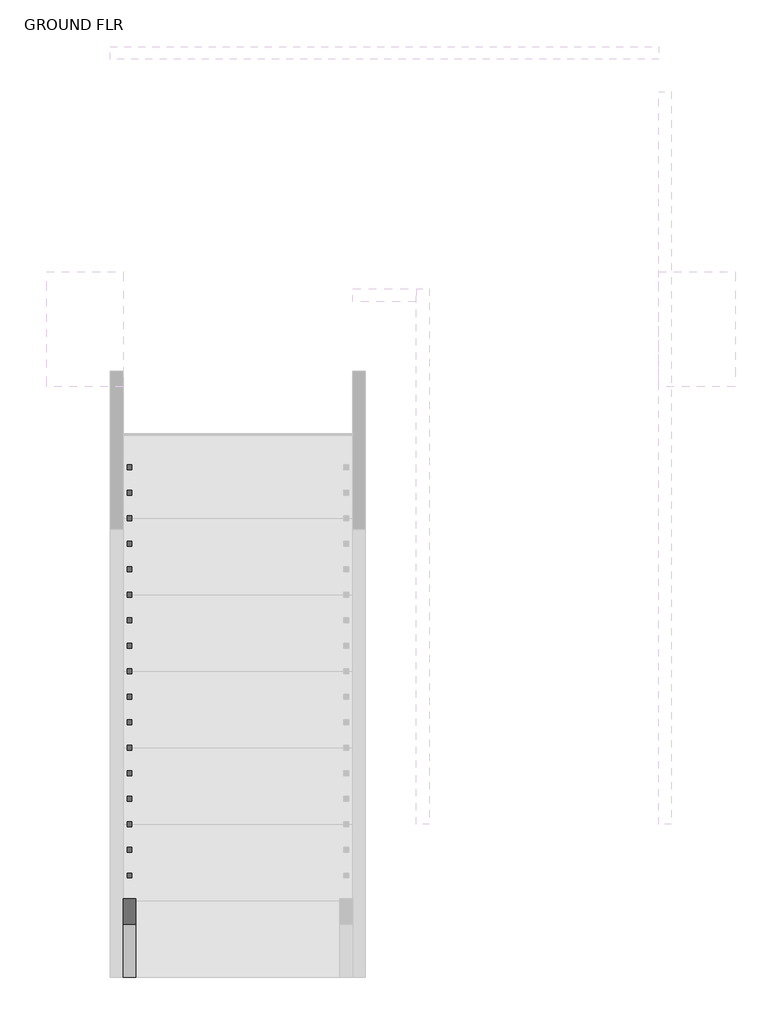
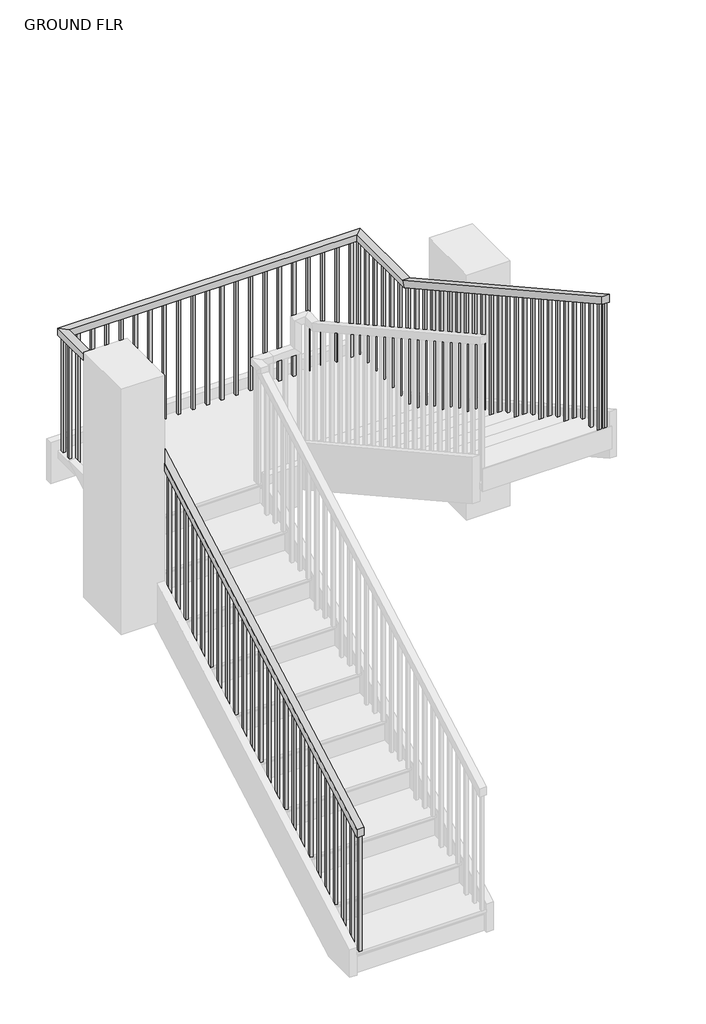
# One storey, part 2 of 4: 1 railing.
"""IFC4 building model written with IfcOpenShell, lengths in millimetres."""

from ifc_helpers import new_model, si_unit, frame, origin, place, context, project, spatial, polyline, outline, extrude, faceted_brep, element, save

model = new_model("IFC4")

# Units and contexts
model_context = context("Model", 3, world=origin())
ifc_project = project(units=[si_unit("LENGTHUNIT", "METRE", prefix="MILLI")], contexts=[model_context])

# Site, building, storey
site = spatial("IfcSite", under=ifc_project)
building = spatial("IfcBuilding", under=site)
storey = spatial("IfcBuildingStorey", under=building, Name="GROUND FLR", Elevation=304.8)

# Railing
placement = place(None, origin())
element("IfcRailing", 1, ObjectType="Handrail - Rectangular", at=placement, inside=storey, context=model_context, shape_type="SolidModel", body=[
    faceted_brep([(-992.1175798, -12221.8061634, 1388.5333333), (-992.1175798, -12221.8061634, 1330.420221), (-941.3175798, -12221.8061634, 1330.420221), (-941.3175798, -12221.8061634, 1388.5333333), (-992.1175798, -9478.6061634, 2912.5333333), (-992.1175798, -9465.4425611, 2861.7333333), (-941.3175798, -9465.4425611, 2861.7333333), (-941.3175798, -9478.6061634, 2912.5333333), (-992.1175798, -8564.2061634, 2912.5333333), (-992.1175798, -8564.2061634, 2861.7333333), (-941.3175798, -8615.0061634, 2861.7333333), (-941.3175798, -8615.0061634, 2912.5333333), (1141.4824202, -8564.2061634, 2912.5333333), (1141.4824202, -8564.2061634, 2861.7333333), (1090.6824202, -8615.0061634, 2861.7333333), (1090.6824202, -8615.0061634, 2912.5333333), (1141.4824202, -9173.8061634, 2912.5333333), (1141.4824202, -9186.9697656, 2861.7333333), (1090.6824202, -9186.9697656, 2861.7333333), (1090.6824202, -9173.8061634, 2912.5333333), (1141.4824202, -11612.2061634, 4267.2), (1090.6824202, -11612.2061634, 4267.2), (1090.6824202, -11612.2061634, 4209.0868876), (1141.4824202, -11612.2061634, 4209.0868876)], [[[0, 1, 2, 3]], [[1, 0, 4, 5]], [[2, 1, 5, 6]], [[3, 2, 6, 7]], [[0, 3, 7, 4]], [[5, 4, 8, 9]], [[6, 5, 9, 10]], [[7, 6, 10, 11]], [[4, 7, 11, 8]], [[9, 8, 12, 13]], [[10, 9, 13, 14]], [[11, 10, 14, 15]], [[8, 11, 15, 12]], [[13, 12, 16, 17]], [[14, 13, 17, 18]], [[15, 14, 18, 19]], [[12, 15, 19, 16]], [[20, 21, 22, 23]], [[17, 16, 20, 23]], [[18, 17, 23, 22]], [[19, 18, 22, 21]], [[16, 19, 21, 20]]]),
    extrude(outline(polyline([(-11526.4811634, 4161.4618876), (-11526.4811634, 3183.4666667), (-11545.5311634, 3183.4666667), (-11545.5311634, 4172.045221), (-11526.4811634, 4161.4618876)])), frame((1106.5574202, 0.0, 0.0), z_axis=(1.0, 0.0, 0.0), x_axis=(0.0, 1.0, 0.0)), (0.0, 0.0, 1.0), 19.05),
    extrude(outline(polyline([(-11424.8811634, 4105.0174432), (-11424.8811634, 3183.4666667), (-11443.9311634, 3183.4666667), (-11443.9311634, 4115.6007765), (-11424.8811634, 4105.0174432)])), frame((1106.5574202, 0.0, 0.0), z_axis=(1.0, 0.0, 0.0), x_axis=(0.0, 1.0, 0.0)), (0.0, 0.0, 1.0), 19.05),
    extrude(outline(polyline([(-11323.2811634, 4048.5729988), (-11323.2811634, 3183.4666667), (-11342.3311634, 3183.4666667), (-11342.3311634, 4059.1563321), (-11323.2811634, 4048.5729988)])), frame((1106.5574202, 0.0, 0.0), z_axis=(1.0, 0.0, 0.0), x_axis=(0.0, 1.0, 0.0)), (0.0, 0.0, 1.0), 19.05),
    extrude(outline(polyline([(-11221.6811634, 3992.1285543), (-11221.6811634, 3014.1333333), (-11240.7311634, 3014.1333333), (-11240.7311634, 4002.7118876), (-11221.6811634, 3992.1285543)])), frame((1106.5574202, 0.0, 0.0), z_axis=(1.0, 0.0, 0.0), x_axis=(0.0, 1.0, 0.0)), (0.0, 0.0, 1.0), 19.05),
    extrude(outline(polyline([(-11120.0811634, 3935.6841099), (-11120.0811634, 3014.1333333), (-11139.1311634, 3014.1333333), (-11139.1311634, 3946.2674432), (-11120.0811634, 3935.6841099)])), frame((1106.5574202, 0.0, 0.0), z_axis=(1.0, 0.0, 0.0), x_axis=(0.0, 1.0, 0.0)), (0.0, 0.0, 1.0), 19.05),
    extrude(outline(polyline([(-11018.4811634, 3879.2396654), (-11018.4811634, 3014.1333333), (-11037.5311634, 3014.1333333), (-11037.5311634, 3889.8229988), (-11018.4811634, 3879.2396654)])), frame((1106.5574202, 0.0, 0.0), z_axis=(1.0, 0.0, 0.0), x_axis=(0.0, 1.0, 0.0)), (0.0, 0.0, 1.0), 19.05),
    extrude(outline(polyline([(-10916.8811634, 3822.795221), (-10916.8811634, 2844.8), (-10935.9311634, 2844.8), (-10935.9311634, 3833.3785543), (-10916.8811634, 3822.795221)])), frame((1106.5574202, 0.0, 0.0), z_axis=(1.0, 0.0, 0.0), x_axis=(0.0, 1.0, 0.0)), (0.0, 0.0, 1.0), 19.05),
    extrude(outline(polyline([(-10815.2811634, 3766.3507765), (-10815.2811634, 2844.8), (-10834.3311634, 2844.8), (-10834.3311634, 3776.9341099), (-10815.2811634, 3766.3507765)])), frame((1106.5574202, 0.0, 0.0), z_axis=(1.0, 0.0, 0.0), x_axis=(0.0, 1.0, 0.0)), (0.0, 0.0, 1.0), 19.05),
    extrude(outline(polyline([(-10713.6811634, 3709.9063321), (-10713.6811634, 2844.8), (-10732.7311634, 2844.8), (-10732.7311634, 3720.4896654), (-10713.6811634, 3709.9063321)])), frame((1106.5574202, 0.0, 0.0), z_axis=(1.0, 0.0, 0.0), x_axis=(0.0, 1.0, 0.0)), (0.0, 0.0, 1.0), 19.05),
    extrude(outline(polyline([(-10612.0811634, 3653.4618876), (-10612.0811634, 2675.4666667), (-10631.1311634, 2675.4666667), (-10631.1311634, 3664.045221), (-10612.0811634, 3653.4618876)])), frame((1106.5574202, 0.0, 0.0), z_axis=(1.0, 0.0, 0.0), x_axis=(0.0, 1.0, 0.0)), (0.0, 0.0, 1.0), 19.05),
    extrude(outline(polyline([(-10510.4811634, 3597.0174432), (-10510.4811634, 2675.4666667), (-10529.5311634, 2675.4666667), (-10529.5311634, 3607.6007765), (-10510.4811634, 3597.0174432)])), frame((1106.5574202, 0.0, 0.0), z_axis=(1.0, 0.0, 0.0), x_axis=(0.0, 1.0, 0.0)), (0.0, 0.0, 1.0), 19.05),
    extrude(outline(polyline([(-10408.8811634, 3540.5729988), (-10408.8811634, 2675.4666667), (-10427.9311634, 2675.4666667), (-10427.9311634, 3551.1563321), (-10408.8811634, 3540.5729988)])), frame((1106.5574202, 0.0, 0.0), z_axis=(1.0, 0.0, 0.0), x_axis=(0.0, 1.0, 0.0)), (0.0, 0.0, 1.0), 19.05),
    extrude(outline(polyline([(-10307.2811634, 3484.1285543), (-10307.2811634, 2506.1333333), (-10326.3311634, 2506.1333333), (-10326.3311634, 3494.7118876), (-10307.2811634, 3484.1285543)])), frame((1106.5574202, 0.0, 0.0), z_axis=(1.0, 0.0, 0.0), x_axis=(0.0, 1.0, 0.0)), (0.0, 0.0, 1.0), 19.05),
    extrude(outline(polyline([(-10205.6811634, 3427.6841099), (-10205.6811634, 2506.1333333), (-10224.7311634, 2506.1333333), (-10224.7311634, 3438.2674432), (-10205.6811634, 3427.6841099)])), frame((1106.5574202, 0.0, 0.0), z_axis=(1.0, 0.0, 0.0), x_axis=(0.0, 1.0, 0.0)), (0.0, 0.0, 1.0), 19.05),
    extrude(outline(polyline([(-10104.0811634, 3371.2396654), (-10104.0811634, 2506.1333333), (-10123.1311634, 2506.1333333), (-10123.1311634, 3381.8229988), (-10104.0811634, 3371.2396654)])), frame((1106.5574202, 0.0, 0.0), z_axis=(1.0, 0.0, 0.0), x_axis=(0.0, 1.0, 0.0)), (0.0, 0.0, 1.0), 19.05),
    extrude(outline(polyline([(-10002.4811634, 3314.795221), (-10002.4811634, 2336.8), (-10021.5311634, 2336.8), (-10021.5311634, 3325.3785543), (-10002.4811634, 3314.795221)])), frame((1106.5574202, 0.0, 0.0), z_axis=(1.0, 0.0, 0.0), x_axis=(0.0, 1.0, 0.0)), (0.0, 0.0, 1.0), 19.05),
    extrude(outline(polyline([(-9900.8811634, 3258.3507765), (-9900.8811634, 2336.8), (-9919.9311634, 2336.8), (-9919.9311634, 3268.9341099), (-9900.8811634, 3258.3507765)])), frame((1106.5574202, 0.0, 0.0), z_axis=(1.0, 0.0, 0.0), x_axis=(0.0, 1.0, 0.0)), (0.0, 0.0, 1.0), 19.05),
    extrude(outline(polyline([(-9799.2811634, 3201.9063321), (-9799.2811634, 2336.8), (-9818.3311634, 2336.8), (-9818.3311634, 3212.4896654), (-9799.2811634, 3201.9063321)])), frame((1106.5574202, 0.0, 0.0), z_axis=(1.0, 0.0, 0.0), x_axis=(0.0, 1.0, 0.0)), (0.0, 0.0, 1.0), 19.05),
    extrude(outline(polyline([(-9697.6811634, 3145.4618876), (-9697.6811634, 2167.4666667), (-9716.7311634, 2167.4666667), (-9716.7311634, 3156.045221), (-9697.6811634, 3145.4618876)])), frame((1106.5574202, 0.0, 0.0), z_axis=(1.0, 0.0, 0.0), x_axis=(0.0, 1.0, 0.0)), (0.0, 0.0, 1.0), 19.05),
    extrude(outline(polyline([(-9596.0811634, 3089.0174432), (-9596.0811634, 2167.4666667), (-9615.1311634, 2167.4666667), (-9615.1311634, 3099.6007765), (-9596.0811634, 3089.0174432)])), frame((1106.5574202, 0.0, 0.0), z_axis=(1.0, 0.0, 0.0), x_axis=(0.0, 1.0, 0.0)), (0.0, 0.0, 1.0), 19.05),
    extrude(outline(polyline([(-9494.4811634, 3032.5729988), (-9494.4811634, 2167.4666667), (-9513.5311634, 2167.4666667), (-9513.5311634, 3043.1563321), (-9494.4811634, 3032.5729988)])), frame((1106.5574202, 0.0, 0.0), z_axis=(1.0, 0.0, 0.0), x_axis=(0.0, 1.0, 0.0)), (0.0, 0.0, 1.0), 19.05),
    extrude(outline(polyline([(-9392.8811634, 2976.1285543), (-9392.8811634, 1998.1333333), (-9411.9311634, 1998.1333333), (-9411.9311634, 2986.7118876), (-9392.8811634, 2976.1285543)])), frame((1106.5574202, 0.0, 0.0), z_axis=(1.0, 0.0, 0.0), x_axis=(0.0, 1.0, 0.0)), (0.0, 0.0, 1.0), 19.05),
    extrude(outline(polyline([(-9291.2811634, 2919.6841099), (-9291.2811634, 1998.1333333), (-9310.3311634, 1998.1333333), (-9310.3311634, 2930.2674432), (-9291.2811634, 2919.6841099)])), frame((1106.5574202, 0.0, 0.0), z_axis=(1.0, 0.0, 0.0), x_axis=(0.0, 1.0, 0.0)), (0.0, 0.0, 1.0), 19.05),
    extrude(outline(polyline([(-9189.6811634, 2863.2396654), (-9189.6811634, 1998.1333333), (-9208.7311634, 1998.1333333), (-9208.7311634, 2873.8229988), (-9189.6811634, 2863.2396654)])), frame((1106.5574202, 0.0, 0.0), z_axis=(1.0, 0.0, 0.0), x_axis=(0.0, 1.0, 0.0)), (0.0, 0.0, 1.0), 19.05),
    extrude(outline(polyline([(1125.6074202, -9088.0811634), (1125.6074202, -9107.1311634), (1106.5574202, -9107.1311634), (1106.5574202, -9088.0811634), (1125.6074202, -9088.0811634)])), frame((0.0, 0.0, 1998.1333333), z_axis=(0.0, 0.0, 1.0), x_axis=(1.0, 0.0, 0.0)), (0.0, 0.0, 1.0), 863.6),
    extrude(outline(polyline([(1125.6074202, -8986.4811634), (1125.6074202, -9005.5311634), (1106.5574202, -9005.5311634), (1106.5574202, -8986.4811634), (1125.6074202, -8986.4811634)])), frame((0.0, 0.0, 1998.1333333), z_axis=(0.0, 0.0, 1.0), x_axis=(1.0, 0.0, 0.0)), (0.0, 0.0, 1.0), 863.6),
    extrude(outline(polyline([(1125.6074202, -8884.8811634), (1125.6074202, -8903.9311634), (1106.5574202, -8903.9311634), (1106.5574202, -8884.8811634), (1125.6074202, -8884.8811634)])), frame((0.0, 0.0, 1998.1333333), z_axis=(0.0, 0.0, 1.0), x_axis=(1.0, 0.0, 0.0)), (0.0, 0.0, 1.0), 863.6),
    extrude(outline(polyline([(1125.6074202, -8783.2811634), (1125.6074202, -8802.3311634), (1106.5574202, -8802.3311634), (1106.5574202, -8783.2811634), (1125.6074202, -8783.2811634)])), frame((0.0, 0.0, 1998.1333333), z_axis=(0.0, 0.0, 1.0), x_axis=(1.0, 0.0, 0.0)), (0.0, 0.0, 1.0), 863.6),
    extrude(outline(polyline([(1125.6074202, -8681.6811634), (1125.6074202, -8700.7311634), (1106.5574202, -8700.7311634), (1106.5574202, -8681.6811634), (1125.6074202, -8681.6811634)])), frame((0.0, 0.0, 1998.1333333), z_axis=(0.0, 0.0, 1.0), x_axis=(1.0, 0.0, 0.0)), (0.0, 0.0, 1.0), 863.6),
    extrude(outline(polyline([(1055.7574202, -8580.0811634), (1074.8074202, -8580.0811634), (1074.8074202, -8599.1311634), (1055.7574202, -8599.1311634), (1055.7574202, -8580.0811634)])), frame((0.0, 0.0, 1998.1333333), z_axis=(0.0, 0.0, 1.0), x_axis=(1.0, 0.0, 0.0)), (0.0, 0.0, 1.0), 863.6),
    extrude(outline(polyline([(954.1574202, -8580.0811634), (973.2074202, -8580.0811634), (973.2074202, -8599.1311634), (954.1574202, -8599.1311634), (954.1574202, -8580.0811634)])), frame((0.0, 0.0, 1998.1333333), z_axis=(0.0, 0.0, 1.0), x_axis=(1.0, 0.0, 0.0)), (0.0, 0.0, 1.0), 863.6),
    extrude(outline(polyline([(852.5574202, -8580.0811634), (871.6074202, -8580.0811634), (871.6074202, -8599.1311634), (852.5574202, -8599.1311634), (852.5574202, -8580.0811634)])), frame((0.0, 0.0, 1998.1333333), z_axis=(0.0, 0.0, 1.0), x_axis=(1.0, 0.0, 0.0)), (0.0, 0.0, 1.0), 863.6),
    extrude(outline(polyline([(750.9574202, -8580.0811634), (770.0074202, -8580.0811634), (770.0074202, -8599.1311634), (750.9574202, -8599.1311634), (750.9574202, -8580.0811634)])), frame((0.0, 0.0, 1998.1333333), z_axis=(0.0, 0.0, 1.0), x_axis=(1.0, 0.0, 0.0)), (0.0, 0.0, 1.0), 863.6),
    extrude(outline(polyline([(649.3574202, -8580.0811634), (668.4074202, -8580.0811634), (668.4074202, -8599.1311634), (649.3574202, -8599.1311634), (649.3574202, -8580.0811634)])), frame((0.0, 0.0, 1998.1333333), z_axis=(0.0, 0.0, 1.0), x_axis=(1.0, 0.0, 0.0)), (0.0, 0.0, 1.0), 863.6),
    extrude(outline(polyline([(547.7574202, -8580.0811634), (566.8074202, -8580.0811634), (566.8074202, -8599.1311634), (547.7574202, -8599.1311634), (547.7574202, -8580.0811634)])), frame((0.0, 0.0, 1998.1333333), z_axis=(0.0, 0.0, 1.0), x_axis=(1.0, 0.0, 0.0)), (0.0, 0.0, 1.0), 863.6),
    extrude(outline(polyline([(446.1574202, -8580.0811634), (465.2074202, -8580.0811634), (465.2074202, -8599.1311634), (446.1574202, -8599.1311634), (446.1574202, -8580.0811634)])), frame((0.0, 0.0, 1998.1333333), z_axis=(0.0, 0.0, 1.0), x_axis=(1.0, 0.0, 0.0)), (0.0, 0.0, 1.0), 863.6),
    extrude(outline(polyline([(344.5574202, -8580.0811634), (363.6074202, -8580.0811634), (363.6074202, -8599.1311634), (344.5574202, -8599.1311634), (344.5574202, -8580.0811634)])), frame((0.0, 0.0, 1998.1333333), z_axis=(0.0, 0.0, 1.0), x_axis=(1.0, 0.0, 0.0)), (0.0, 0.0, 1.0), 863.6),
    extrude(outline(polyline([(242.9574202, -8580.0811634), (262.0074202, -8580.0811634), (262.0074202, -8599.1311634), (242.9574202, -8599.1311634), (242.9574202, -8580.0811634)])), frame((0.0, 0.0, 1998.1333333), z_axis=(0.0, 0.0, 1.0), x_axis=(1.0, 0.0, 0.0)), (0.0, 0.0, 1.0), 863.6),
    extrude(outline(polyline([(141.3574202, -8580.0811634), (160.4074202, -8580.0811634), (160.4074202, -8599.1311634), (141.3574202, -8599.1311634), (141.3574202, -8580.0811634)])), frame((0.0, 0.0, 1998.1333333), z_axis=(0.0, 0.0, 1.0), x_axis=(1.0, 0.0, 0.0)), (0.0, 0.0, 1.0), 863.6),
    extrude(outline(polyline([(39.7574202, -8580.0811634), (58.8074202, -8580.0811634), (58.8074202, -8599.1311634), (39.7574202, -8599.1311634), (39.7574202, -8580.0811634)])), frame((0.0, 0.0, 1998.1333333), z_axis=(0.0, 0.0, 1.0), x_axis=(1.0, 0.0, 0.0)), (0.0, 0.0, 1.0), 863.6),
    extrude(outline(polyline([(-61.8425798, -8580.0811634), (-42.7925798, -8580.0811634), (-42.7925798, -8599.1311634), (-61.8425798, -8599.1311634), (-61.8425798, -8580.0811634)])), frame((0.0, 0.0, 1998.1333333), z_axis=(0.0, 0.0, 1.0), x_axis=(1.0, 0.0, 0.0)), (0.0, 0.0, 1.0), 863.6),
    extrude(outline(polyline([(-163.4425798, -8580.0811634), (-144.3925798, -8580.0811634), (-144.3925798, -8599.1311634), (-163.4425798, -8599.1311634), (-163.4425798, -8580.0811634)])), frame((0.0, 0.0, 1998.1333333), z_axis=(0.0, 0.0, 1.0), x_axis=(1.0, 0.0, 0.0)), (0.0, 0.0, 1.0), 863.6),
    extrude(outline(polyline([(-265.0425798, -8580.0811634), (-245.9925798, -8580.0811634), (-245.9925798, -8599.1311634), (-265.0425798, -8599.1311634), (-265.0425798, -8580.0811634)])), frame((0.0, 0.0, 1998.1333333), z_axis=(0.0, 0.0, 1.0), x_axis=(1.0, 0.0, 0.0)), (0.0, 0.0, 1.0), 863.6),
    extrude(outline(polyline([(-366.6425798, -8580.0811634), (-347.5925798, -8580.0811634), (-347.5925798, -8599.1311634), (-366.6425798, -8599.1311634), (-366.6425798, -8580.0811634)])), frame((0.0, 0.0, 1998.1333333), z_axis=(0.0, 0.0, 1.0), x_axis=(1.0, 0.0, 0.0)), (0.0, 0.0, 1.0), 863.6),
    extrude(outline(polyline([(-468.2425798, -8580.0811634), (-449.1925798, -8580.0811634), (-449.1925798, -8599.1311634), (-468.2425798, -8599.1311634), (-468.2425798, -8580.0811634)])), frame((0.0, 0.0, 1998.1333333), z_axis=(0.0, 0.0, 1.0), x_axis=(1.0, 0.0, 0.0)), (0.0, 0.0, 1.0), 863.6),
    extrude(outline(polyline([(-569.8425798, -8580.0811634), (-550.7925798, -8580.0811634), (-550.7925798, -8599.1311634), (-569.8425798, -8599.1311634), (-569.8425798, -8580.0811634)])), frame((0.0, 0.0, 1998.1333333), z_axis=(0.0, 0.0, 1.0), x_axis=(1.0, 0.0, 0.0)), (0.0, 0.0, 1.0), 863.6),
    extrude(outline(polyline([(-671.4425798, -8580.0811634), (-652.3925798, -8580.0811634), (-652.3925798, -8599.1311634), (-671.4425798, -8599.1311634), (-671.4425798, -8580.0811634)])), frame((0.0, 0.0, 1998.1333333), z_axis=(0.0, 0.0, 1.0), x_axis=(1.0, 0.0, 0.0)), (0.0, 0.0, 1.0), 863.6),
    extrude(outline(polyline([(-773.0425798, -8580.0811634), (-753.9925798, -8580.0811634), (-753.9925798, -8599.1311634), (-773.0425798, -8599.1311634), (-773.0425798, -8580.0811634)])), frame((0.0, 0.0, 1998.1333333), z_axis=(0.0, 0.0, 1.0), x_axis=(1.0, 0.0, 0.0)), (0.0, 0.0, 1.0), 863.6),
    extrude(outline(polyline([(-874.6425798, -8580.0811634), (-855.5925798, -8580.0811634), (-855.5925798, -8599.1311634), (-874.6425798, -8599.1311634), (-874.6425798, -8580.0811634)])), frame((0.0, 0.0, 1998.1333333), z_axis=(0.0, 0.0, 1.0), x_axis=(1.0, 0.0, 0.0)), (0.0, 0.0, 1.0), 863.6),
    extrude(outline(polyline([(-976.2425798, -8675.3311634), (-976.2425798, -8656.2811634), (-957.1925798, -8656.2811634), (-957.1925798, -8675.3311634), (-976.2425798, -8675.3311634)])), frame((0.0, 0.0, 1998.1333333), z_axis=(0.0, 0.0, 1.0), x_axis=(1.0, 0.0, 0.0)), (0.0, 0.0, 1.0), 863.6),
    extrude(outline(polyline([(-976.2425798, -8776.9311634), (-976.2425798, -8757.8811634), (-957.1925798, -8757.8811634), (-957.1925798, -8776.9311634), (-976.2425798, -8776.9311634)])), frame((0.0, 0.0, 1998.1333333), z_axis=(0.0, 0.0, 1.0), x_axis=(1.0, 0.0, 0.0)), (0.0, 0.0, 1.0), 863.6),
    extrude(outline(polyline([(-976.2425798, -8878.5311634), (-976.2425798, -8859.4811634), (-957.1925798, -8859.4811634), (-957.1925798, -8878.5311634), (-976.2425798, -8878.5311634)])), frame((0.0, 0.0, 1998.1333333), z_axis=(0.0, 0.0, 1.0), x_axis=(1.0, 0.0, 0.0)), (0.0, 0.0, 1.0), 863.6),
    extrude(outline(polyline([(-976.2425798, -8980.1311634), (-976.2425798, -8961.0811634), (-957.1925798, -8961.0811634), (-957.1925798, -8980.1311634), (-976.2425798, -8980.1311634)])), frame((0.0, 0.0, 1998.1333333), z_axis=(0.0, 0.0, 1.0), x_axis=(1.0, 0.0, 0.0)), (0.0, 0.0, 1.0), 863.6),
    extrude(outline(polyline([(-976.2425798, -9081.7311634), (-976.2425798, -9062.6811634), (-957.1925798, -9062.6811634), (-957.1925798, -9081.7311634), (-976.2425798, -9081.7311634)])), frame((0.0, 0.0, 1998.1333333), z_axis=(0.0, 0.0, 1.0), x_axis=(1.0, 0.0, 0.0)), (0.0, 0.0, 1.0), 863.6),
    extrude(outline(polyline([(-976.2425798, -9183.3311634), (-976.2425798, -9164.2811634), (-957.1925798, -9164.2811634), (-957.1925798, -9183.3311634), (-976.2425798, -9183.3311634)])), frame((0.0, 0.0, 1998.1333333), z_axis=(0.0, 0.0, 1.0), x_axis=(1.0, 0.0, 0.0)), (0.0, 0.0, 1.0), 863.6),
    extrude(outline(polyline([(-976.2425798, -9284.9311634), (-976.2425798, -9265.8811634), (-957.1925798, -9265.8811634), (-957.1925798, -9284.9311634), (-976.2425798, -9284.9311634)])), frame((0.0, 0.0, 1998.1333333), z_axis=(0.0, 0.0, 1.0), x_axis=(1.0, 0.0, 0.0)), (0.0, 0.0, 1.0), 863.6),
    extrude(outline(polyline([(-976.2425798, -9386.5311634), (-976.2425798, -9367.4811634), (-957.1925798, -9367.4811634), (-957.1925798, -9386.5311634), (-976.2425798, -9386.5311634)])), frame((0.0, 0.0, 1998.1333333), z_axis=(0.0, 0.0, 1.0), x_axis=(1.0, 0.0, 0.0)), (0.0, 0.0, 1.0), 863.6),
    extrude(outline(polyline([(-9469.0811634, 2859.7118876), (-9469.0811634, 1998.1333333), (-9488.1311634, 1998.1333333), (-9488.1311634, 2849.1285543), (-9469.0811634, 2859.7118876)])), frame((-976.2425798, 0.0, 0.0), z_axis=(1.0, 0.0, 0.0), x_axis=(0.0, 1.0, 0.0)), (0.0, 0.0, 1.0), 19.05),
    extrude(outline(polyline([(-9570.6811634, 2803.2674432), (-9570.6811634, 1828.8), (-9589.7311634, 1828.8), (-9589.7311634, 2792.6841099), (-9570.6811634, 2803.2674432)])), frame((-976.2425798, 0.0, 0.0), z_axis=(1.0, 0.0, 0.0), x_axis=(0.0, 1.0, 0.0)), (0.0, 0.0, 1.0), 19.05),
    extrude(outline(polyline([(-9672.2811634, 2746.8229988), (-9672.2811634, 1828.8), (-9691.3311634, 1828.8), (-9691.3311634, 2736.2396654), (-9672.2811634, 2746.8229988)])), frame((-976.2425798, 0.0, 0.0), z_axis=(1.0, 0.0, 0.0), x_axis=(0.0, 1.0, 0.0)), (0.0, 0.0, 1.0), 19.05),
    extrude(outline(polyline([(-9773.8811634, 2690.3785543), (-9773.8811634, 1828.8), (-9792.9311634, 1828.8), (-9792.9311634, 2679.795221), (-9773.8811634, 2690.3785543)])), frame((-976.2425798, 0.0, 0.0), z_axis=(1.0, 0.0, 0.0), x_axis=(0.0, 1.0, 0.0)), (0.0, 0.0, 1.0), 19.05),
    extrude(outline(polyline([(-9875.4811634, 2633.9341099), (-9875.4811634, 1659.4666667), (-9894.5311634, 1659.4666667), (-9894.5311634, 2623.3507765), (-9875.4811634, 2633.9341099)])), frame((-976.2425798, 0.0, 0.0), z_axis=(1.0, 0.0, 0.0), x_axis=(0.0, 1.0, 0.0)), (0.0, 0.0, 1.0), 19.05),
    extrude(outline(polyline([(-9977.0811634, 2577.4896654), (-9977.0811634, 1659.4666667), (-9996.1311634, 1659.4666667), (-9996.1311634, 2566.9063321), (-9977.0811634, 2577.4896654)])), frame((-976.2425798, 0.0, 0.0), z_axis=(1.0, 0.0, 0.0), x_axis=(0.0, 1.0, 0.0)), (0.0, 0.0, 1.0), 19.05),
    extrude(outline(polyline([(-10078.6811634, 2521.045221), (-10078.6811634, 1659.4666667), (-10097.7311634, 1659.4666667), (-10097.7311634, 2510.4618876), (-10078.6811634, 2521.045221)])), frame((-976.2425798, 0.0, 0.0), z_axis=(1.0, 0.0, 0.0), x_axis=(0.0, 1.0, 0.0)), (0.0, 0.0, 1.0), 19.05),
    extrude(outline(polyline([(-10180.2811634, 2464.6007765), (-10180.2811634, 1490.1333333), (-10199.3311634, 1490.1333333), (-10199.3311634, 2454.0174432), (-10180.2811634, 2464.6007765)])), frame((-976.2425798, 0.0, 0.0), z_axis=(1.0, 0.0, 0.0), x_axis=(0.0, 1.0, 0.0)), (0.0, 0.0, 1.0), 19.05),
    extrude(outline(polyline([(-10281.8811634, 2408.1563321), (-10281.8811634, 1490.1333333), (-10300.9311634, 1490.1333333), (-10300.9311634, 2397.5729988), (-10281.8811634, 2408.1563321)])), frame((-976.2425798, 0.0, 0.0), z_axis=(1.0, 0.0, 0.0), x_axis=(0.0, 1.0, 0.0)), (0.0, 0.0, 1.0), 19.05),
    extrude(outline(polyline([(-10383.4811634, 2351.7118876), (-10383.4811634, 1490.1333333), (-10402.5311634, 1490.1333333), (-10402.5311634, 2341.1285543), (-10383.4811634, 2351.7118876)])), frame((-976.2425798, 0.0, 0.0), z_axis=(1.0, 0.0, 0.0), x_axis=(0.0, 1.0, 0.0)), (0.0, 0.0, 1.0), 19.05),
    extrude(outline(polyline([(-10485.0811634, 2295.2674432), (-10485.0811634, 1320.8), (-10504.1311634, 1320.8), (-10504.1311634, 2284.6841099), (-10485.0811634, 2295.2674432)])), frame((-976.2425798, 0.0, 0.0), z_axis=(1.0, 0.0, 0.0), x_axis=(0.0, 1.0, 0.0)), (0.0, 0.0, 1.0), 19.05),
    extrude(outline(polyline([(-10586.6811634, 2238.8229988), (-10586.6811634, 1320.8), (-10605.7311634, 1320.8), (-10605.7311634, 2228.2396654), (-10586.6811634, 2238.8229988)])), frame((-976.2425798, 0.0, 0.0), z_axis=(1.0, 0.0, 0.0), x_axis=(0.0, 1.0, 0.0)), (0.0, 0.0, 1.0), 19.05),
    extrude(outline(polyline([(-10688.2811634, 2182.3785543), (-10688.2811634, 1320.8), (-10707.3311634, 1320.8), (-10707.3311634, 2171.795221), (-10688.2811634, 2182.3785543)])), frame((-976.2425798, 0.0, 0.0), z_axis=(1.0, 0.0, 0.0), x_axis=(0.0, 1.0, 0.0)), (0.0, 0.0, 1.0), 19.05),
    extrude(outline(polyline([(-10789.8811634, 2125.9341099), (-10789.8811634, 1151.4666667), (-10808.9311634, 1151.4666667), (-10808.9311634, 2115.3507765), (-10789.8811634, 2125.9341099)])), frame((-976.2425798, 0.0, 0.0), z_axis=(1.0, 0.0, 0.0), x_axis=(0.0, 1.0, 0.0)), (0.0, 0.0, 1.0), 19.05),
    extrude(outline(polyline([(-10891.4811634, 2069.4896654), (-10891.4811634, 1151.4666667), (-10910.5311634, 1151.4666667), (-10910.5311634, 2058.9063321), (-10891.4811634, 2069.4896654)])), frame((-976.2425798, 0.0, 0.0), z_axis=(1.0, 0.0, 0.0), x_axis=(0.0, 1.0, 0.0)), (0.0, 0.0, 1.0), 19.05),
    extrude(outline(polyline([(-10993.0811634, 2013.045221), (-10993.0811634, 1151.4666667), (-11012.1311634, 1151.4666667), (-11012.1311634, 2002.4618876), (-10993.0811634, 2013.045221)])), frame((-976.2425798, 0.0, 0.0), z_axis=(1.0, 0.0, 0.0), x_axis=(0.0, 1.0, 0.0)), (0.0, 0.0, 1.0), 19.05),
    extrude(outline(polyline([(-11094.6811634, 1956.6007765), (-11094.6811634, 982.1333333), (-11113.7311634, 982.1333333), (-11113.7311634, 1946.0174432), (-11094.6811634, 1956.6007765)])), frame((-976.2425798, 0.0, 0.0), z_axis=(1.0, 0.0, 0.0), x_axis=(0.0, 1.0, 0.0)), (0.0, 0.0, 1.0), 19.05),
    extrude(outline(polyline([(-11196.2811634, 1900.1563321), (-11196.2811634, 982.1333333), (-11215.3311634, 982.1333333), (-11215.3311634, 1889.5729988), (-11196.2811634, 1900.1563321)])), frame((-976.2425798, 0.0, 0.0), z_axis=(1.0, 0.0, 0.0), x_axis=(0.0, 1.0, 0.0)), (0.0, 0.0, 1.0), 19.05),
    extrude(outline(polyline([(-11297.8811634, 1843.7118876), (-11297.8811634, 982.1333333), (-11316.9311634, 982.1333333), (-11316.9311634, 1833.1285543), (-11297.8811634, 1843.7118876)])), frame((-976.2425798, 0.0, 0.0), z_axis=(1.0, 0.0, 0.0), x_axis=(0.0, 1.0, 0.0)), (0.0, 0.0, 1.0), 19.05),
    extrude(outline(polyline([(-11399.4811634, 1787.2674432), (-11399.4811634, 812.8), (-11418.5311634, 812.8), (-11418.5311634, 1776.6841099), (-11399.4811634, 1787.2674432)])), frame((-976.2425798, 0.0, 0.0), z_axis=(1.0, 0.0, 0.0), x_axis=(0.0, 1.0, 0.0)), (0.0, 0.0, 1.0), 19.05),
    extrude(outline(polyline([(-11501.0811634, 1730.8229988), (-11501.0811634, 812.8), (-11520.1311634, 812.8), (-11520.1311634, 1720.2396654), (-11501.0811634, 1730.8229988)])), frame((-976.2425798, 0.0, 0.0), z_axis=(1.0, 0.0, 0.0), x_axis=(0.0, 1.0, 0.0)), (0.0, 0.0, 1.0), 19.05),
    extrude(outline(polyline([(-11602.6811634, 1674.3785543), (-11602.6811634, 812.8), (-11621.7311634, 812.8), (-11621.7311634, 1663.795221), (-11602.6811634, 1674.3785543)])), frame((-976.2425798, 0.0, 0.0), z_axis=(1.0, 0.0, 0.0), x_axis=(0.0, 1.0, 0.0)), (0.0, 0.0, 1.0), 19.05),
    extrude(outline(polyline([(-11704.2811634, 1617.9341099), (-11704.2811634, 643.4666667), (-11723.3311634, 643.4666667), (-11723.3311634, 1607.3507765), (-11704.2811634, 1617.9341099)])), frame((-976.2425798, 0.0, 0.0), z_axis=(1.0, 0.0, 0.0), x_axis=(0.0, 1.0, 0.0)), (0.0, 0.0, 1.0), 19.05),
    extrude(outline(polyline([(-11805.8811634, 1561.4896654), (-11805.8811634, 643.4666667), (-11824.9311634, 643.4666667), (-11824.9311634, 1550.9063321), (-11805.8811634, 1561.4896654)])), frame((-976.2425798, 0.0, 0.0), z_axis=(1.0, 0.0, 0.0), x_axis=(0.0, 1.0, 0.0)), (0.0, 0.0, 1.0), 19.05),
    extrude(outline(polyline([(-11907.4811634, 1505.045221), (-11907.4811634, 643.4666667), (-11926.5311634, 643.4666667), (-11926.5311634, 1494.4618876), (-11907.4811634, 1505.045221)])), frame((-976.2425798, 0.0, 0.0), z_axis=(1.0, 0.0, 0.0), x_axis=(0.0, 1.0, 0.0)), (0.0, 0.0, 1.0), 19.05),
    extrude(outline(polyline([(-12009.0811634, 1448.6007765), (-12009.0811634, 474.1333333), (-12028.1311634, 474.1333333), (-12028.1311634, 1438.0174432), (-12009.0811634, 1448.6007765)])), frame((-976.2425798, 0.0, 0.0), z_axis=(1.0, 0.0, 0.0), x_axis=(0.0, 1.0, 0.0)), (0.0, 0.0, 1.0), 19.05),
    extrude(outline(polyline([(-12110.6811634, 1392.1563321), (-12110.6811634, 474.1333333), (-12129.7311634, 474.1333333), (-12129.7311634, 1381.5729988), (-12110.6811634, 1392.1563321)])), frame((-976.2425798, 0.0, 0.0), z_axis=(1.0, 0.0, 0.0), x_axis=(0.0, 1.0, 0.0)), (0.0, 0.0, 1.0), 19.05),
    extrude(outline(polyline([(1106.5574202, -8580.0811634), (1125.6074202, -8580.0811634), (1125.6074202, -8599.1311634), (1106.5574202, -8599.1311634), (1106.5574202, -8580.0811634)])), frame((0.0, 0.0, 1998.1333333), z_axis=(0.0, 0.0, 1.0), x_axis=(1.0, 0.0, 0.0)), (0.0, 0.0, 1.0), 863.6),
    extrude(outline(polyline([(-976.2425798, -8599.1311634), (-976.2425798, -8580.0811634), (-957.1925798, -8580.0811634), (-957.1925798, -8599.1311634), (-976.2425798, -8599.1311634)])), frame((0.0, 0.0, 1998.1333333), z_axis=(0.0, 0.0, 1.0), x_axis=(1.0, 0.0, 0.0)), (0.0, 0.0, 1.0), 863.6),
    extrude(outline(polyline([(-11593.1561634, 4198.5035543), (-11593.1561634, 3183.4666667), (-11612.2061634, 3183.4666667), (-11612.2061634, 4209.0868876), (-11593.1561634, 4198.5035543)])), frame((1106.5574202, 0.0, 0.0), z_axis=(1.0, 0.0, 0.0), x_axis=(0.0, 1.0, 0.0)), (0.0, 0.0, 1.0), 19.05),
    extrude(outline(polyline([(-12202.7561634, 1341.0035543), (-12202.7561634, 474.1333333), (-12221.8061634, 474.1333333), (-12221.8061634, 1330.420221), (-12202.7561634, 1341.0035543)])), frame((-976.2425798, 0.0, 0.0), z_axis=(1.0, 0.0, 0.0), x_axis=(0.0, 1.0, 0.0)), (0.0, 0.0, 1.0), 19.05),
])

save(model, "model.ifc")

# Revit data of these elements
# Type "Handrail - Rectangular"
#   Assembly Code = "C2010400"
#   built-in parameter 1008612 = 0.0416667 (stored number, unit not read)
#   built-in parameter 1008611 = 0.0416667 (stored number, unit not read)
#   built-in parameter 1008609 = 0.333333 (stored number, unit not read)
#   built-in parameter 1008604 = 0.166667 (stored number, unit not read)
#   built-in parameter 1008603 = 0.166667 (stored number, unit not read)
#   Railing Height = 3' - 0"
#   built-in parameter 1008630 = 2
#   built-in parameter 1008610 = 2
#   built-in parameter 1008618 = Baluster - Square : 3/4"
# Element 1 (IfcRailing, "Handrail - Rectangular")
#   Phase Created = New Construction
